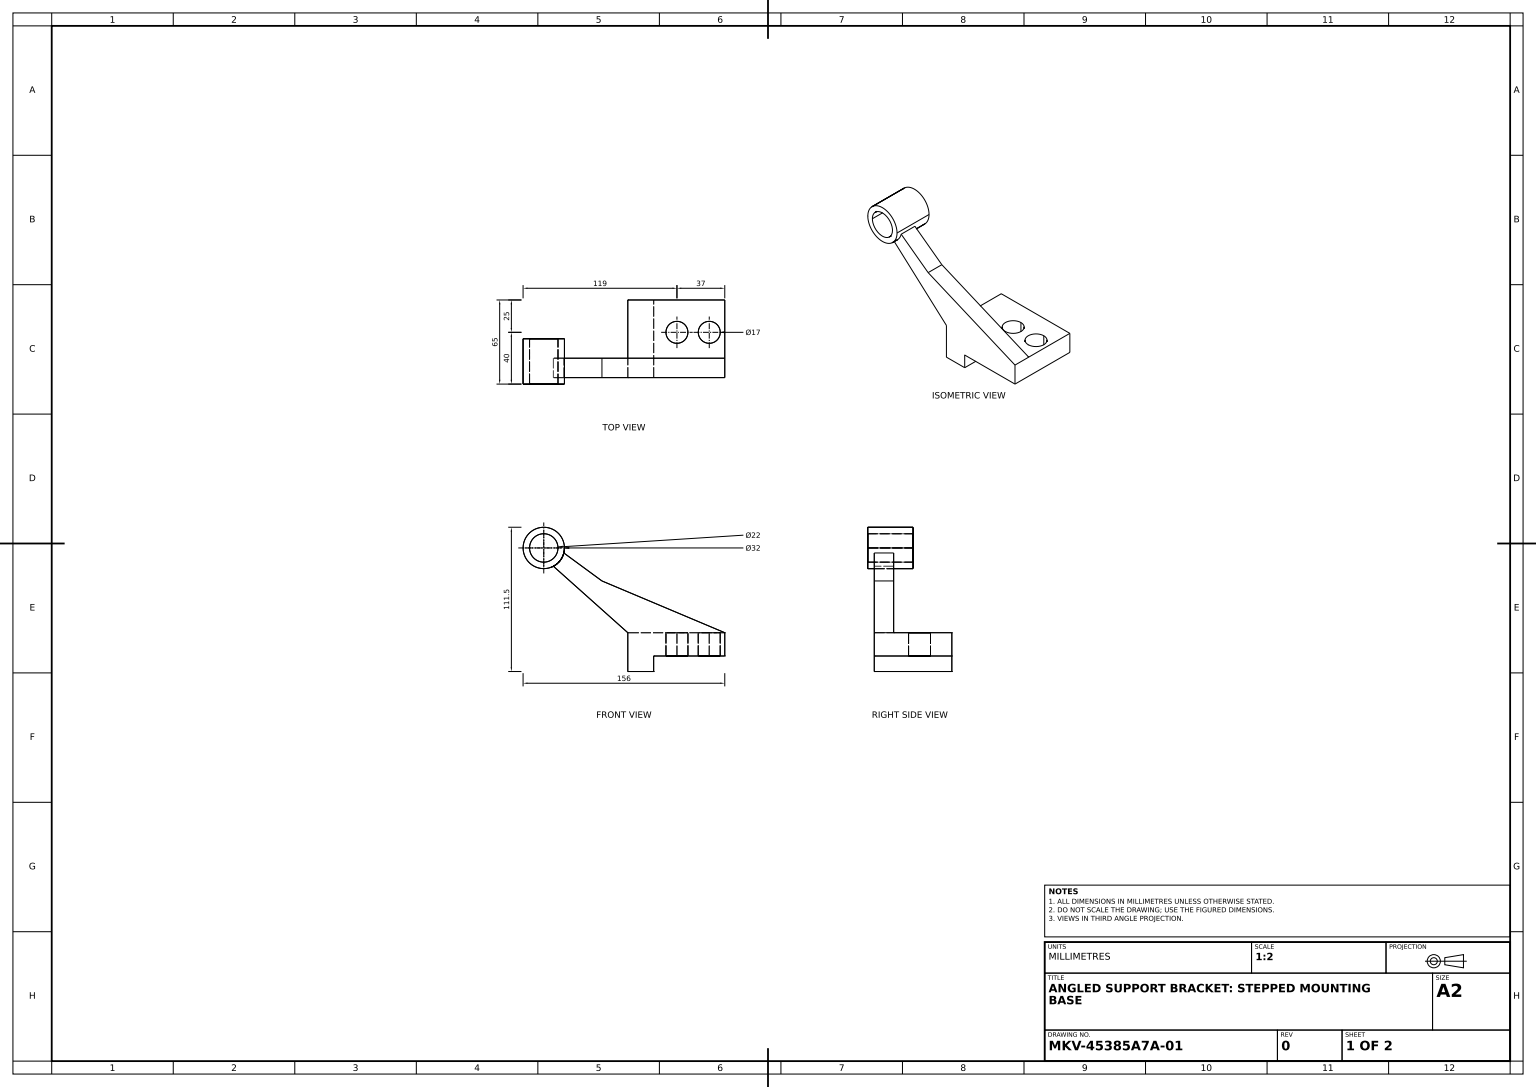
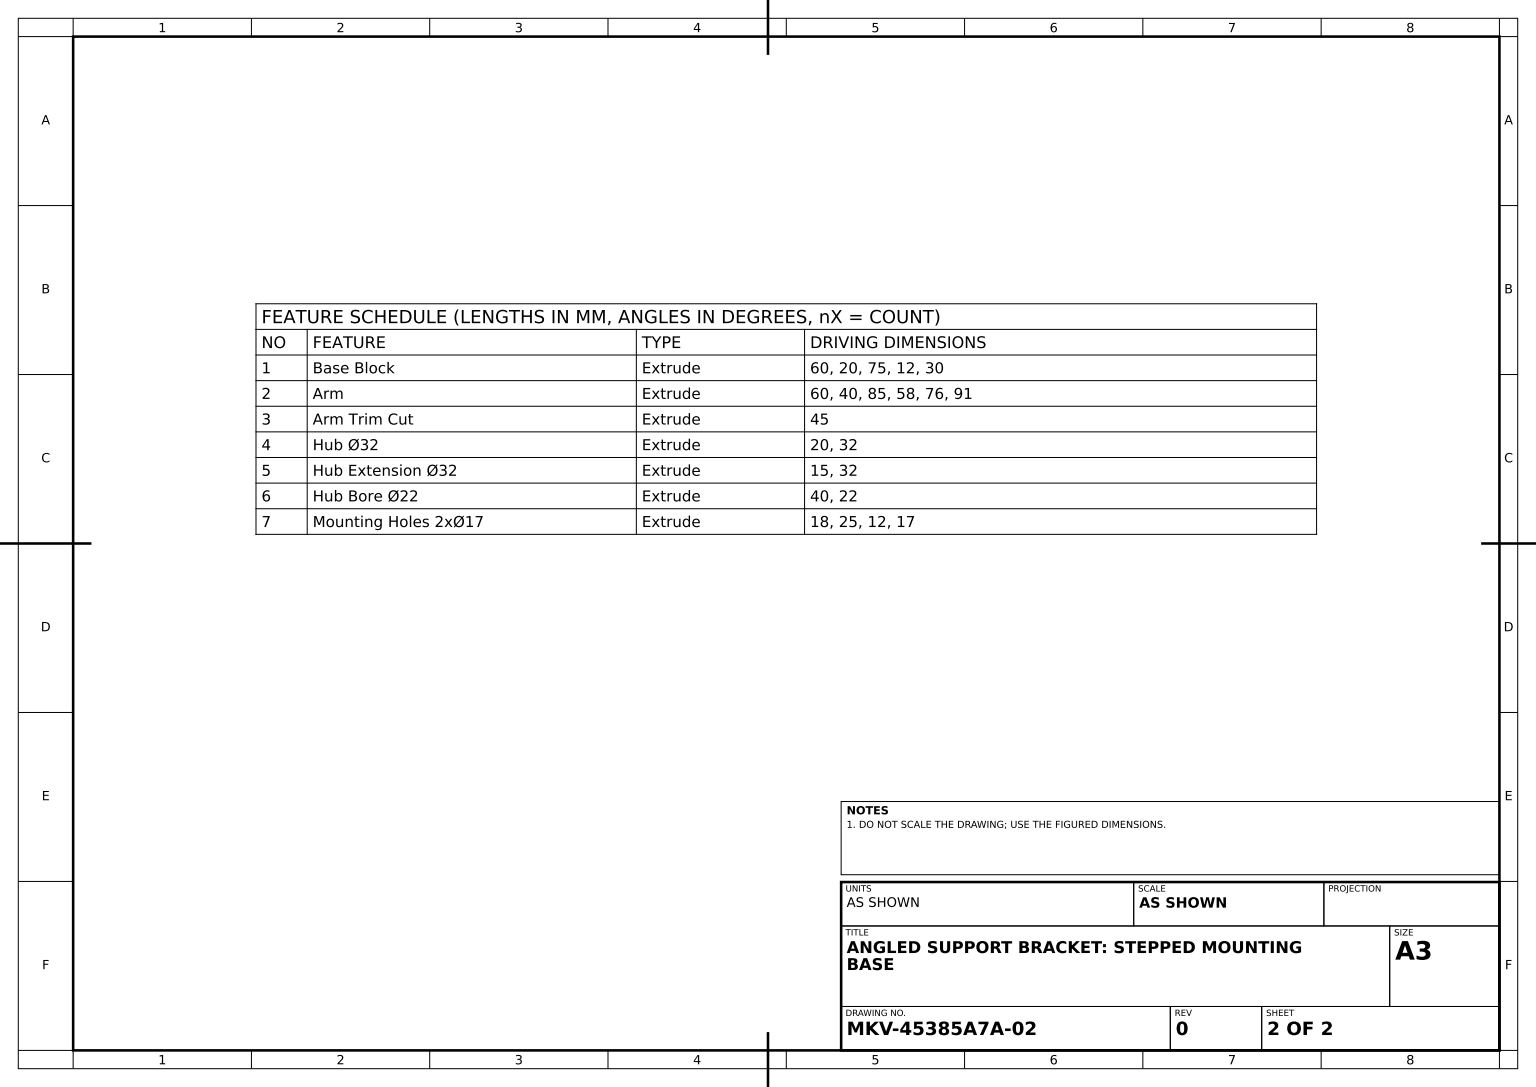
SolidWorks part; units mm, degrees
material "Plain Carbon Steel"
ref_plane "Front Plane" through (0, 0, 0) normal (0, 0, 1) x (1, 0, 0)
ref_plane "Top Plane" through (0, 0, 0) normal (0, 1, 0) x (1, 0, 0)
ref_plane "Right Plane" through (0, 0, 0) normal (1, 0, 0) x (0, 0, -1)
sketch "Base Profile Sketch" plane through (0, 0, 0) normal (0, 0, 1) x (1, 0, 0)
  line L0 (0, 0) -> (-75, 0)
  line L1 (-75, 0) -> (-75, -30)
  line L2 (-75, -30) -> (-55, -30)
  line L3 (-55, -30) -> (-55, -18)
  line L4 (-55, -18) -> (0, -18)
  line L5 (0, -18) -> (0, 0)
  dimension "D1" = 20
  dimension "D2" = 75
  dimension "D3" = 12
  dimension "D4" = 30
extrude "Base Block" add sketch "Base Profile Sketch" along normal blind 60
sketch "Arm Profile Sketch" plane through (0, 0, 0) normal (0, 0, -1) x (-1, 0, 0)
  line L1 (0, 0) -> (75, 0)
  line L4 (0, 0) -> (95, 40)
  line L5 (75, 0) -> (140, 58)
  line L6 (140, 58) -> (140, 73)
  line L7 (140, 73) -> (95, 40)
  line L8 (55, -30) -> (55, -18) construction
  line L9 (55, -18) -> (0, -18) construction
  dimension "D1" = 40
  dimension "D2" = 85
  dimension "D3" = 58
  dimension "D4" = 76
  dimension "D5" = 91
extrude "Arm" add sketch "Arm Profile Sketch" against normal blind 60
sketch "Arm Trim Sketch" plane through (0, 0, 0) normal (0, 0, -1) x (-1, 0, 0)
  line L0 (0, 0) -> (95, 40)
  line L1 (95, 40) -> (140, 73)
  line L2 (140, 73) -> (140, 58)
  line L3 (140, 58) -> (75, 0)
  line L4 (75, 0) -> (0, 0)
extrude "Arm Trim Cut" cut sketch "Arm Trim Sketch" against normal blind 45
sketch "Hub Sketch Ø32" plane through (0, 0, 45) normal (0, 0, -1) x (-1, 0, 0)
  line L0 (140, 58) -> (140, 73) construction
  circle A0 centre (140, 65.5) radius 16
  dimension "D1" = 32
  dimension "D2" = 32
extrude "Hub Ø32" add sketch "Hub Sketch Ø32" against normal blind 20
sketch "Hub Extension Sketch Ø32" plane through (0, 0, 45) normal (0, 0, -1) x (-1, 0, 0)
  circle A0 centre (140, 65.5) radius 16
  dimension "D1" = 32
  dimension "D2" = 32
extrude "Hub Extension Ø32" add sketch "Hub Extension Sketch Ø32" along normal blind 15
sketch "Bore Sketch Ø22" plane through (0, 0, 30) normal (0, 0, -1) x (-1, 0, 0)
  circle A0 centre (140, 65.5) radius 11
  dimension "D1" = 22
  dimension "D2" = 22
extrude "Hub Bore Ø22" cut sketch "Bore Sketch Ø22" against normal blind 40
sketch "Mounting Holes Sketch" plane through (0, 0, 0) normal (0, 1, 0) x (1, 0, 0)
  line L0 (0, 0) -> (-75, 0) construction
  line L1 (0, -45) -> (0, 0) construction
  circle A0 centre (-12, -25) radius 8.5
  circle A1 centre (-37, -25) radius 8.5
  dimension "D1" = 17
  dimension "D4" = 17
  dimension "D6" = 17
  dimension "D2" = 25
  dimension "D3" = 12
  dimension "D5" = 25
extrude "Mounting Holes 2xØ17" cut sketch "Mounting Holes Sketch" against normal blind 18
